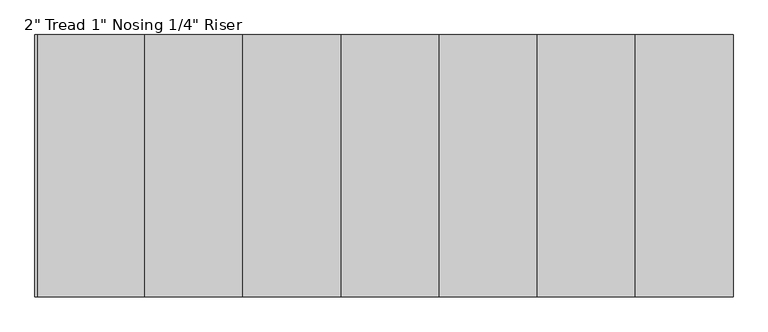
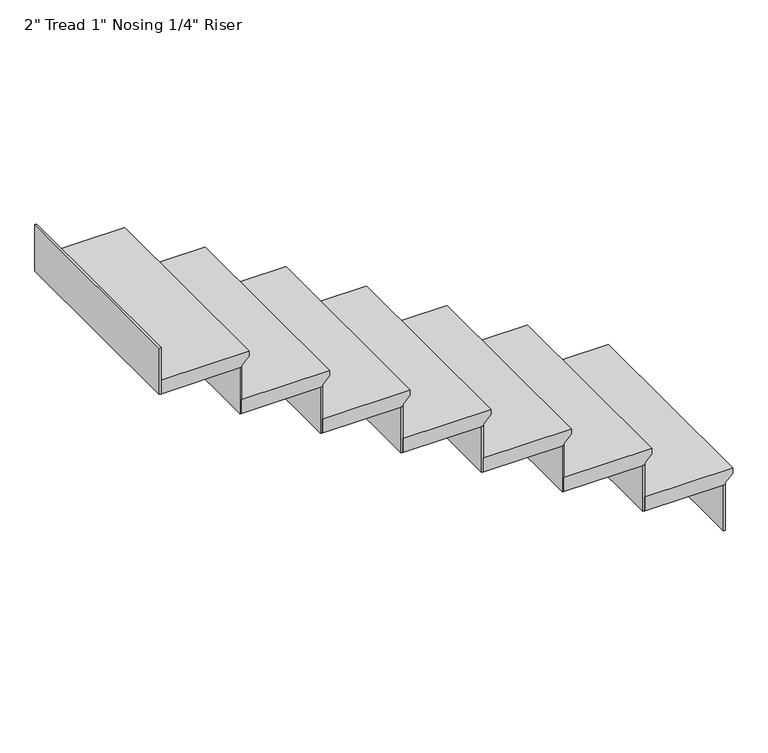
"""IFC4 building model written with IfcOpenShell, lengths in millimetres: stair flight geometry."""

from ifc_helpers import new_model, si_unit, frame, origin, place, context, project, spatial, polyline, outline, extrude, source, transform, mapped, element, save


def stair_flight_9de2ea67(model_context):
    return source(origin(), model_context, "Body", "SweptSolid", [
        extrude(outline(polyline([(1524.0, -6546.9655018), (1524.0, -6851.7655018), (1473.2, -6851.7655018), (1473.2, -6572.3655018), (1479.55, -6572.3655018), (1504.95, -6546.9655018), (1524.0, -6546.9655018)])), frame((0.0, 601.995692, 0.0), z_axis=(0.0, 1.0, 0.0), x_axis=(0.0, 0.0, 1.0)), (0.0, 0.0, 1.0), 746.8619448),
        extrude(outline(polyline([(-6578.7155018, 1348.8576368), (-6572.3655018, 1348.8576368), (-6572.3655018, 601.995692), (-6578.7155018, 601.995692), (-6578.7155018, 1348.8576368)])), frame((0.0, 0.0, 1303.8666667), z_axis=(0.0, 0.0, 1.0), x_axis=(1.0, 0.0, 0.0)), (0.0, 0.0, 1.0), 169.3333333),
        extrude(outline(polyline([(-8534.5155018, 1348.8576368), (-8528.1655018, 1348.8576368), (-8528.1655018, 601.995692), (-8534.5155018, 601.995692), (-8534.5155018, 1348.8576368)])), frame((0.0, 0.0, 2489.2), z_axis=(0.0, 0.0, 1.0), x_axis=(1.0, 0.0, 0.0)), (0.0, 0.0, 1.0), 169.3333333),
        extrude(outline(polyline([(-6858.1155018, 1348.8576368), (-6851.7655018, 1348.8576368), (-6851.7655018, 601.995692), (-6858.1155018, 601.995692), (-6858.1155018, 1348.8576368)])), frame((0.0, 0.0, 1473.2), z_axis=(0.0, 0.0, 1.0), x_axis=(1.0, 0.0, 0.0)), (0.0, 0.0, 1.0), 169.3333333),
        extrude(outline(polyline([(1693.3333333, -6826.3655018), (1693.3333333, -7131.1655018), (1642.5333333, -7131.1655018), (1642.5333333, -6851.7655018), (1648.8833333, -6851.7655018), (1674.2833333, -6826.3655018), (1693.3333333, -6826.3655018)])), frame((0.0, 601.995692, 0.0), z_axis=(0.0, 1.0, 0.0), x_axis=(0.0, 0.0, 1.0)), (0.0, 0.0, 1.0), 746.8619448),
        extrude(outline(polyline([(-7137.5155018, 1348.8576368), (-7131.1655018, 1348.8576368), (-7131.1655018, 601.995692), (-7137.5155018, 601.995692), (-7137.5155018, 1348.8576368)])), frame((0.0, 0.0, 1642.5333333), z_axis=(0.0, 0.0, 1.0), x_axis=(1.0, 0.0, 0.0)), (0.0, 0.0, 1.0), 169.3333333),
        extrude(outline(polyline([(1862.6666667, -7105.7655018), (1862.6666667, -7410.5655018), (1811.8666667, -7410.5655018), (1811.8666667, -7131.1655018), (1818.2166667, -7131.1655018), (1843.6166667, -7105.7655018), (1862.6666667, -7105.7655018)])), frame((0.0, 601.995692, 0.0), z_axis=(0.0, 1.0, 0.0), x_axis=(0.0, 0.0, 1.0)), (0.0, 0.0, 1.0), 746.8619448),
        extrude(outline(polyline([(-7416.9155018, 1348.8576368), (-7410.5655018, 1348.8576368), (-7410.5655018, 601.995692), (-7416.9155018, 601.995692), (-7416.9155018, 1348.8576368)])), frame((0.0, 0.0, 1811.8666667), z_axis=(0.0, 0.0, 1.0), x_axis=(1.0, 0.0, 0.0)), (0.0, 0.0, 1.0), 169.3333333),
        extrude(outline(polyline([(2032.0, -7385.1655018), (2032.0, -7689.9655018), (1981.2, -7689.9655018), (1981.2, -7410.5655018), (1987.55, -7410.5655018), (2012.95, -7385.1655018), (2032.0, -7385.1655018)])), frame((0.0, 601.995692, 0.0), z_axis=(0.0, 1.0, 0.0), x_axis=(0.0, 0.0, 1.0)), (0.0, 0.0, 1.0), 746.8619448),
        extrude(outline(polyline([(-7696.3155018, 1348.8576368), (-7689.9655018, 1348.8576368), (-7689.9655018, 601.995692), (-7696.3155018, 601.995692), (-7696.3155018, 1348.8576368)])), frame((0.0, 0.0, 1981.2), z_axis=(0.0, 0.0, 1.0), x_axis=(1.0, 0.0, 0.0)), (0.0, 0.0, 1.0), 169.3333333),
        extrude(outline(polyline([(2201.3333333, -7664.5655018), (2201.3333333, -7969.3655018), (2150.5333333, -7969.3655018), (2150.5333333, -7689.9655018), (2156.8833333, -7689.9655018), (2182.2833333, -7664.5655018), (2201.3333333, -7664.5655018)])), frame((0.0, 601.995692, 0.0), z_axis=(0.0, 1.0, 0.0), x_axis=(0.0, 0.0, 1.0)), (0.0, 0.0, 1.0), 746.8619448),
        extrude(outline(polyline([(-7975.7155018, 1348.8576368), (-7969.3655018, 1348.8576368), (-7969.3655018, 601.995692), (-7975.7155018, 601.995692), (-7975.7155018, 1348.8576368)])), frame((0.0, 0.0, 2150.5333333), z_axis=(0.0, 0.0, 1.0), x_axis=(1.0, 0.0, 0.0)), (0.0, 0.0, 1.0), 169.3333333),
        extrude(outline(polyline([(2370.6666667, -7943.9655018), (2370.6666667, -8248.7655018), (2319.8666667, -8248.7655018), (2319.8666667, -7969.3655018), (2326.2166667, -7969.3655018), (2351.6166667, -7943.9655018), (2370.6666667, -7943.9655018)])), frame((0.0, 601.995692, 0.0), z_axis=(0.0, 1.0, 0.0), x_axis=(0.0, 0.0, 1.0)), (0.0, 0.0, 1.0), 746.8619448),
        extrude(outline(polyline([(-8255.1155018, 1348.8576368), (-8248.7655018, 1348.8576368), (-8248.7655018, 601.995692), (-8255.1155018, 601.995692), (-8255.1155018, 1348.8576368)])), frame((0.0, 0.0, 2319.8666667), z_axis=(0.0, 0.0, 1.0), x_axis=(1.0, 0.0, 0.0)), (0.0, 0.0, 1.0), 169.3333333),
        extrude(outline(polyline([(2540.0, -8223.3655018), (2540.0, -8528.1655018), (2489.2, -8528.1655018), (2489.2, -8248.7655018), (2495.55, -8248.7655018), (2520.95, -8223.3655018), (2540.0, -8223.3655018)])), frame((0.0, 601.995692, 0.0), z_axis=(0.0, 1.0, 0.0), x_axis=(0.0, 0.0, 1.0)), (0.0, 0.0, 1.0), 746.8619448),
    ])


if __name__ == "__main__":
    model = new_model("IFC4")
    model_context = context("Model", 3, world=origin())
    ifc_project = project(units=[si_unit("LENGTHUNIT", "METRE", prefix="MILLI")], contexts=[model_context])
    site = spatial("IfcSite", under=ifc_project)
    building = spatial("IfcBuilding", under=site)
    placement = place(None, origin())
    stair_flight_shape = stair_flight_9de2ea67(model_context)
    element("IfcStairFlight", 1, ObjectType="2\" Tread 1\" Nosing 1/4\" Riser", at=placement, inside=building, context=model_context, shape_type="MappedRepresentation", body=[
        mapped(stair_flight_shape, transform((0.0, 0.0, 0.0), x_axis=(1.0, 0.0, 0.0), y_axis=(0.0, 1.0, 0.0), z_axis=(0.0, 0.0, 1.0))),
    ])
    save(model, "model.ifc")
